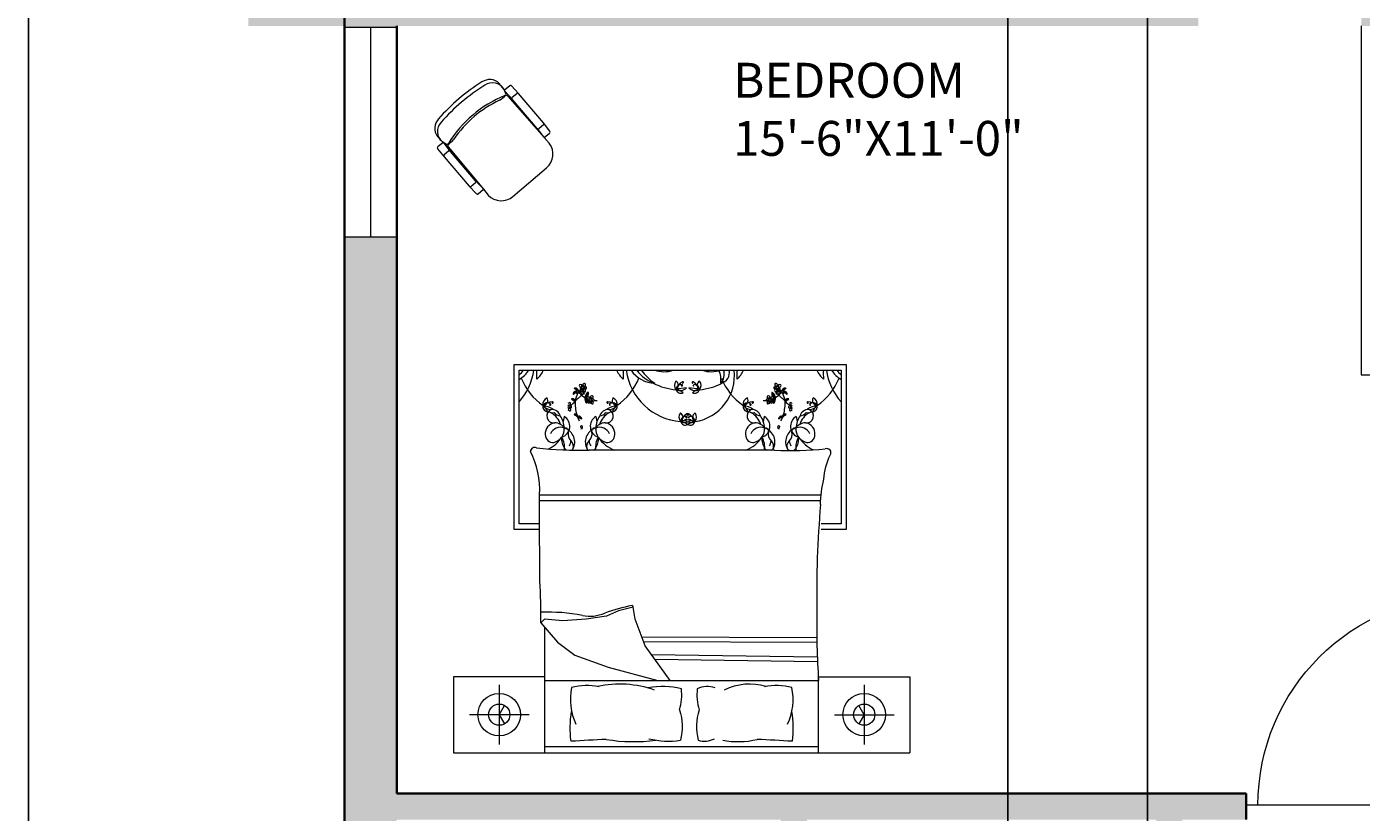
# Model space of a CAD drawing. Units: inches. Extents: x -36 to 442, y -676 to 151.
# Tile 5 of 8: x -36 to 193, y -134 to 1. Entities that reach past the tile are written whole.
import ezdxf

# ---------------------------------------------------------------- set-up
doc = ezdxf.new("R2010")
doc.units = ezdxf.units.IN
doc.header["$MEASUREMENT"] = 0
for name, color, linetype, lineweight in [('A-ANNO-DIMS', 2, 'Continuous', 18), ('A-AREA-IDEN', 7, 'Continuous', 18), ('A-DOOR', 4, 'Continuous', 18), ('A-FLOR-CASE', 32, 'Continuous', 18), ('A-FURN', 9, 'Continuous', 13), ('A-GLAZ', 4, 'Continuous', 13), ('A-WALL', 7, 'Continuous', 35), ('A-WALL-PATT', 8, 'Continuous', 13)]:
    doc.layers.add(name, color=color, linetype=linetype, lineweight=lineweight)
doc.styles.get("Standard").update_dxf_attribs({"font": 'arial.ttf'})
doc.dimstyles.get("Standard").update_dxf_attribs({"dimtxt": 0.18, "dimasz": 0.18, "dimexe": 0.18, "dimexo": 0.0625, "dimgap": 0.09, "dimtad": 0, "dimtih": 1, "dimtoh": 1, "dimdec": 0, "dimzin": 0, "dimdsep": 46, "dimlunit": 3, "dimtxsty": 'Standard', "dimcen": 0.09, "dimadec": 0, "dimazin": 0, "dimtfac": 1, "dimtdec": 0, "dimtofl": 0, "dimtmove": 0, "dimatfit": 3, "dimfxl": 1, "dimtolj": 1, "dimtzin": 0, "dimarcsym": 0})

# ---------------------------------------------------------------- blocks, each defined once
blk = doc.blocks.new('DOOR-SWING-36IN')
for p, q in [((2, 0), (2, 36)), ((3, 0), (3, 36)), ((0, 0), (2, 0)), ((2, 0), (3, 0)), ((3, 0), (38, 0)), ((38, 0), (40, 0))]:
    blk.add_line(p, q)
blk.add_arc((2, 0), 36, 0, 90)
blk = doc.blocks.new('GLAZING-UNIT-36IN')
for p, q in [((0, 36), (0, 0)), ((4.5, 36), (4.5, 0)), ((9, 0), (9, 36))]:
    blk.add_line(p, q)
blk = doc.blocks.new('*D50')
at = {"layer": 'A-ANNO-DIMS', "color": 0, "lineweight": -2, "transparency": 16777216}
for p, q in [((97.44, 113.5), (-35.74, 113.5)), ((-35.56, 113.32), (-35.56, -262.07)), ((-35.56, -637.82), (-35.56, -262.43)), ((18.67, -638), (-35.74, -638))]:
    blk.add_line(p, q, dxfattribs=at)
at = {"layer": 'A-ANNO-DIMS', "color": 0, "transparency": 16777216}
for points in [[(-35.59, 113.32), (-35.53, 113.32), (-35.56, 113.5)], [(-35.59, -637.82), (-35.53, -637.82), (-35.56, -638)]]:
    blk.add_solid(points, dxfattribs=at)
at = {"layer": 'Defpoints', "color": 0, "transparency": 16777216}
for p in [(-35.56, 113.5), (97.5, 113.5), (18.74, -638)]:
    blk.add_point(p, dxfattribs=at)
at = {"layer": 'A-ANNO-DIMS', "color": 0, "transparency": 16777216, "insert": (-35.56, -262.25), "char_height": 0.18, "attachment_point": 5}
blk.add_mtext('\\A1;751.5', dxfattribs=at)
blk = doc.blocks.new('*D63')
at = {"layer": 'A-ANNO-DIMS', "color": 0, "lineweight": -2, "transparency": 16777216}
for p, q in [((132.74, -447.43), (132.74, 151.48)), ((156.74, -471.43), (156.74, 151.48)), ((132.92, 151.3), (144.51, 151.3)), ((156.56, 151.3), (144.96, 151.3))]:
    blk.add_line(p, q, dxfattribs=at)
at = {"layer": 'A-ANNO-DIMS', "color": 0, "transparency": 16777216}
for points in [[(132.92, 151.33), (132.92, 151.27), (132.74, 151.3)], [(156.56, 151.33), (156.56, 151.27), (156.74, 151.3)]]:
    blk.add_solid(points, dxfattribs=at)
at = {"layer": 'Defpoints', "color": 0, "transparency": 16777216}
for p in [(156.74, 151.3), (132.74, -447.5), (156.74, -471.5)]:
    blk.add_point(p, dxfattribs=at)
at = {"layer": 'A-ANNO-DIMS', "color": 0, "transparency": 16777216, "insert": (144.74, 151.3), "char_height": 0.18, "attachment_point": 5}
blk.add_mtext('\\A1;24', dxfattribs=at)

msp = doc.modelspace()

# ---------------------------------------------------------------- hatches: boundary and pattern name
at = {"layer": 'A-WALL-PATT'}
h = msp.add_hatch(color=256, dxfattribs=at)
h.dxf.hatch_style = 1
h.paths.add_polyline_path([(288, 113.503), (193.5, 113.503), (97.5, 113.503), (97.5, 104.864), (106.5, 104.864), (106.5, 104.503), (193.5, 104.503), (193.5, 5.503), (193.5, 1.003), (213.735, 1.003), (213.735, -135.497), (218.235, -135.497), (218.235, 1.003), (251, 1.003), (251, 3.253), (251, 5.503), (198, 5.503), (198, 104.503), (279, 104.503), (279, 104.209), (288, 104.209)])
h.paths.add_polyline_path([(378.735, 81.646), (362.235, 81.646), (288, 81.646), (288, 80.209), (279, 80.209), (279, 5.503), (279, 1.003), (353.235, 1.003), (353.235, 0.242), (362.235, 0.242), (362.235, 5.503), (288, 5.503), (288, 77.146), (362.235, 77.146), (374.235, 77.146), (374.235, 5.503), (362.235, 5.503), (362.235, 1.003), (374.235, 1.003), (378.735, 1.003), (378.735, 5.503), (378.735, 77.146)])
h.paths.add_polyline_path([(362.235, -35.758), (353.235, -35.758), (353.235, -196.997), (218.235, -196.997), (213.735, -196.997), (213.735, -205.997), (218.235, -205.997), (378.735, -205.997), (378.735, -205.779), (387.735, -205.779), (387.735, -202.472), (387.735, -196.997), (378.735, -196.997), (362.235, -196.997)])
h.paths.add_polyline_path([(218.235, -175.497), (215.985, -175.497), (213.735, -175.497), (213.735, -196.997), (218.235, -196.997)], flags=17)
h.paths.add_polyline_path([(158.235, -201.497), (98.235, -201.497), (98.235, -205.997), (158.235, -205.997)])
h.paths.add_polyline_path([(173.735, -130.997), (27.735, -130.997), (27.735, -35.267), (18.735, -35.267), (18.735, -138.68), (27.735, -138.68), (27.735, -135.497), (93.735, -135.497), (93.735, -201.497), (98.235, -201.497), (98.235, -135.497), (158.235, -135.497), (158.235, -173.497), (160.739, -173.497), (162.735, -173.497), (162.735, -135.497), (173.735, -135.497), (173.735, -133.017)])
h.paths.add_polyline_path([(98.235, -201.497), (93.735, -201.497), (93.735, -205.997), (98.235, -205.997)])
h.paths.add_polyline_path([(162.735, -201.497), (158.235, -201.497), (158.235, -205.997), (162.735, -205.997)])
h.paths.add_polyline_path([(63.735, -205.997), (63.735, -201.497), (27.735, -201.497), (27.735, -162.68), (18.735, -162.68), (18.735, -210.497), (63.735, -210.497)])
h.paths.add_polyline_path([(65.735, -203.604), (65.735, -201.497), (63.735, -201.497), (63.735, -205.997), (65.735, -205.997)])
h.paths.add_polyline_path([(165.5, 5.503), (106.5, 5.503), (106.5, 80.864), (97.5, 80.864), (97.5, 81.646), (6.735, 81.646), (2.235, 81.646), (2.235, 77.146), (2.235, 5.503), (2.235, 1.003), (6.735, 1.003), (18.735, 1.003), (18.735, 5.503), (6.735, 5.503), (6.735, 77.146), (97.5, 77.146), (97.5, 5.503), (18.735, 5.503), (18.735, 0.733), (27.735, 0.733), (27.735, 1.003), (165.5, 1.003), (165.5, 3.253)])
h.paths.add_polyline_path([(18.735, -201.497), (6.735, -201.497), (2.235, -201.497), (2.235, -210.497), (2.235, -354.497), (2.235, -363.497), (6.735, -363.497), (18.735, -363.497), (18.735, -358.997), (18.735, -354.497), (6.735, -354.497), (6.735, -210.497), (18.735, -210.497)])
h.paths.add_polyline_path([(63.735, -210.497), (54.735, -210.497), (54.735, -240.747), (63.735, -240.747)])
h.paths.add_polyline_path([(63.735, -336.747), (54.735, -336.747), (54.735, -354.497), (18.735, -354.497), (18.735, -358.997), (18.735, -363.497), (104.735, -363.497), (104.735, -361.247), (104.735, -358.997), (63.735, -358.997)])
h.paths.add_polyline_path([(27.735, -448.151), (18.735, -448.151), (18.735, -637.997), (72.735, -637.997), (72.735, -571.997), (183.235, -571.997), (183.235, -562.997), (57.197, -562.997), (51.735, -562.997), (51.735, -567.497), (57.197, -567.497), (63.735, -567.497), (63.735, -571.997), (63.735, -628.997), (27.735, -628.997), (27.735, -475.997), (27.735, -471.497)])
h.paths.add_polyline_path([(27.735, -363.497), (18.735, -363.497), (18.735, -412.151), (27.735, -412.151)])
h.paths.add_polyline_path([(161.235, -358.997), (132.735, -358.997), (132.735, -363.497), (156.735, -363.497), (156.735, -471.497), (51.735, -471.497), (51.735, -475.997), (63.735, -475.997), (63.735, -534.997), (65.985, -534.997), (68.235, -534.997), (68.235, -475.997), (161.235, -475.997)])
h.paths.add_polyline_path([(161.235, -511.997), (173.235, -511.997), (173.235, -502.997), (161.235, -502.997), (161.235, -475.997), (152.235, -475.997), (152.235, -534.997), (156.735, -534.997), (161.235, -534.997)], flags=17)
h.paths.add_polyline_path([(362.235, -502.997), (353.235, -502.997), (213.235, -502.997), (213.235, -507.497), (213.235, -511.997), (362.235, -511.997)])
h.paths.add_polyline_path([(242.235, -548.019), (233.235, -548.019), (233.235, -562.997), (223.235, -562.997), (223.235, -567.497), (223.235, -571.997), (242.235, -571.997)])
h.paths.add_polyline_path([(404.235, -502.997), (399.735, -502.997), (362.235, -502.997), (362.235, -511.997), (399.735, -511.997), (404.235, -511.997)])
h.paths.add_polyline_path([(362.235, -482.123), (353.235, -482.123), (353.235, -502.997), (362.235, -502.997)])
h.paths.add_polyline_path([(404.235, -295.997), (404.235, -286.997), (387.735, -286.997), (387.735, -295.997), (399.735, -295.997), (399.735, -502.997), (404.235, -502.997)])
h.paths.add_polyline_path([(362.235, -355.863), (353.235, -355.863), (353.235, -386.123), (362.235, -386.123)])
h.paths.add_polyline_path([(387.735, -286.997), (378.735, -286.997), (213.735, -286.997), (213.735, -295.997), (353.235, -295.997), (353.235, -295.863), (362.235, -295.863), (362.235, -295.997), (378.735, -295.997), (387.735, -295.997)])
h.paths.add_polyline_path([(387.735, -241.779), (378.735, -241.779), (378.735, -286.997), (387.735, -286.997)])
h.paths.add_polyline_path([(387.735, -175.497), (362.235, -175.497), (362.235, -184.497), (387.735, -184.497)], flags=17)
h.paths.add_polyline_path([(387.735, -184.497), (383.235, -184.497), (383.235, -192.497), (378.735, -192.497), (366.735, -192.497), (366.735, -184.497), (362.235, -184.497), (362.235, -196.997), (378.735, -196.997), (387.735, -196.997)], flags=17)
h.paths.add_polyline_path([(240.604, 40.967), (282.575, 40.967), (282.575, 63.356), (240.604, 63.356)], flags=25)

# ---------------------------------------------------------------- linework, layer by layer
at = {"layer": 'A-FLOR-CASE'}
for p, q in [((193.5, 1.003), (193.5, -58.997)), ((193.5, -58.997), (213.735, -58.997))]:
    msp.add_line(p, q, dxfattribs=at)
at = {"layer": 'A-FURN', "ltscale": 0.03}
for p, q in [((45.926, -9.597), (45.342, -8.918)), ((46.56, -10.788), (46.166, -9.936)), ((47.561, -11.582), (46.359, -10.265)), ((46.834, -11.066), (53.081, -18.212)), ((47.587, -11.252), (48.345, -10.608)), ((51.846, -16.621), (47.561, -11.582)), ((52.934, -16.003), (52.176, -16.647)), ((35.278, -18.653), (34.702, -17.967)), ((51.846, -16.621), (52.686, -17.761)), ((36.353, -19.469), (35.575, -18.944)), ((36.975, -20.585), (35.868, -19.188)), ((36.645, -20.558), (35.888, -21.203)), ((36.583, -19.785), (42.633, -27.098)), ((41.261, -25.624), (36.975, -20.585)), ((40.476, -26.598), (41.234, -25.954)), ((41.261, -25.624), (42.251, -26.636))]:
    msp.add_line(p, q, dxfattribs=at)
at = {"layer": 'A-FURN'}
for p, q in [((47.849, -57.313), (47.849, -85.559)), ((105.014, -57.313), (47.849, -57.313)), ((105.014, -85.559), (105.014, -57.313)), ((48.757, -58.221), (104.105, -58.221)), ((48.757, -84.65), (48.757, -58.221)), ((104.105, -58.221), (104.105, -84.65)), ((56.484, -66.171), (56.311, -67.057)), ((61.964, -66.171), (62.138, -67.057)), ((90.898, -66.171), (90.725, -67.057)), ((96.378, -66.171), (96.551, -67.057)), ((92.623, -71.988), (60.787, -71.988)), ((100.659, -79.69), (52.278, -79.69)), ((100.584, -80.668), (52.278, -80.668)), ((52.282, -84.65), (48.757, -84.65)), ((104.105, -84.65), (100.649, -84.65)), ((47.849, -85.559), (52.284, -85.559)), ((100.665, -85.559), (105.014, -85.559)), ((63.755, -100.545), (60.261, -101.021)), ((65.82, -99.593), (63.755, -100.545)), ((68.361, -98.958), (65.82, -99.593)), ((68.679, -101.021), (68.361, -98.958)), ((53.115, -101.021), (52.479, -101.656)), ((52.479, -101.656), (55.338, -104.989)), ((56.291, -101.339), (53.115, -101.021)), ((53.181, -123.996), (53.181, -102.475)), ((60.261, -101.021), (56.291, -101.339)), ((70.426, -105.624), (68.679, -101.021)), ((55.338, -104.989), (58.356, -107.211)), ((99.951, -104.269), (69.865, -104.146)), ((99.947, -105.074), (70.172, -104.956)), ((58.356, -107.211), (64.073, -109.275)), ((74.722, -111.605), (70.426, -105.624)), ((99.987, -107.543), (71.515, -107.141)), ((64.073, -109.275), (72.623, -111.605)), ((100.018, -108.348), (72.101, -107.956)), ((45.34, -112.339), (45.34, -122.585)), ((53.181, -111.605), (100.228, -111.605)), ((108.069, -112.339), (108.069, -122.585)), ((50.463, -117.462), (40.217, -117.462)), ((102.946, -117.462), (113.192, -117.462)), ((100.228, -122.99), (53.181, -122.99)), ((37.499, -123.996), (115.91, -123.996))]:
    msp.add_line(p, q, dxfattribs=at)
at = {"layer": 'A-FURN', "ltscale": 0.03}
msp.add_lwpolyline([(34.702, -17.967), (34.99, -18.31, 0.029912), (35.457, -18.852, 0.0631929), (35.697, -19.026), (34.781, -19.805, 0.4142136), (34.754, -20.135), (35.861, -21.533), (40.146, -26.571), (40.146, -26.571), (40.146, -26.571), (41.393, -27.845, 0.4142136), (41.723, -27.872), (42.633, -27.098), (43.458, -28.095, 0.4039906), (47.693, -28.333), (53.488, -23.405, 0.4039906), (53.932, -19.186), (53.081, -18.212), (53.991, -17.438, 0.4142136), (54.018, -17.108), (52.96, -15.673), (48.675, -10.634), (47.473, -9.318, 0.4142136), (47.143, -9.291), (46.227, -10.07, 0.0631952), (46.094, -9.806, 0.029912), (45.634, -9.257), (45.342, -8.918, 0.1969574), (43.912, -8.235, 0.1563962), (42.376, -8.633, 0.0348091), (38.409, -11.547, 0.0348091), (34.897, -14.994, 0.1563962), (34.258, -16.446, 0.1969574)], format="xyb", close=True, dxfattribs=at)
at = {"layer": 'A-FURN'}
for points in [[(52.315, -94.476, -0.0012423), (52.278, -79.599, 0.1272016), (50.706, -72.184)], [(100.563, -81.286, -0.0561118), (101.132, -76.972, -0.0953413), (102.234, -72.816)], [(57.685, -122.042, -0.0748968), (57.78, -116.92, 0.4728166)], [(76.337, -116.634, -0.1409896), (76.494, -121.859, -0.2352448)], [(79.686, -116.634, 0.1409896), (79.529, -121.859, 0.2352448)], [(95.724, -122.042, 0.0748968), (95.629, -116.92, -0.4728166)]]:
    msp.add_lwpolyline(points, format="xyb", dxfattribs=at)
for points in [[(53.181, -110.928), (37.499, -110.928), (37.499, -123.996)], [(100.228, -123.996), (100.228, -110.928), (115.91, -110.928), (115.91, -123.996)], [(45.34, -117.462), (46.255, -115.878)], [(108.069, -117.462), (107.154, -115.878)], [(45.34, -117.462), (46.255, -119.046)], [(108.069, -117.462), (107.154, -119.046)]]:
    msp.add_lwpolyline(points, dxfattribs=at)
for centre, radius in [((59.708, -61.225), 0.2), ((93.154, -61.225), 0.2), ((61.014, -63.33), 0.2), ((91.848, -63.33), 0.2), ((45.34, -117.462), 3.659), ((108.069, -117.462), 3.659), ((45.34, -117.462), 1.83), ((108.069, -117.462), 1.83)]:
    msp.add_circle(centre, radius, dxfattribs=at)
at = {"layer": 'A-FURN', "ltscale": 0.03}
for centre, radius, start, end in [((44.163, -11.096), 2.314, 30.08252, 124.53168), ((61.256, -38.41), 34.534, 122.20561, 138.55381), ((53.845, -29.695), 20.169, 111.96244, 148.79994), ((43.335, -8.119), 4.205, 299.29135, 318.21611), ((46.281, -10.698), 0.293, 274.06172, 341.95455), ((46.527, -11.322), 0.399, 39.82995, 99.60618), ((47.739, -11.43), 0.234, 130.38119, 220.38119), ((48.497, -10.786), 0.234, 40.38119, 130.38119), ((53.845, -29.695), 19.803, 115.26646, 145.49592), ((37.041, -17.154), 2.314, 136.2307, 230.67985), ((52.782, -15.825), 0.234, 310.38119, 40.38119), ((52.024, -16.469), 0.234, 220.38119, 310.38119), ((36.308, -19.18), 0.293, 278.80783, 346.70066), ((36.884, -19.523), 0.399, 161.15619, 220.93242), ((34.235, -15.858), 4.205, 302.54626, 321.47102), ((36.797, -20.737), 0.234, 40.38119, 130.38119), ((36.039, -21.381), 0.234, 130.38119, 220.38119), ((40.325, -26.42), 0.234, 220.38119, 310.38119), ((41.082, -25.775), 0.234, 310.38119, 40.38119)]:
    msp.add_arc(centre, radius, start, end, dxfattribs=at)
at = {"layer": 'A-FURN'}
for centre, radius, start, end in [((44.476, -54.54), 6.218, 313.51858, 323.69643), ((46.271, -55.47), 4.989, 299.88843, 326.53828), ((41.134, -56.842), 10.239, 318.1144, 352.25504), ((58.652, -55.829), 10.239, 201.40921, 235.61345), ((49.065, -56.625), 4.163, 311.04544, 337.44526), ((37.661, -58.862), 14.167, 356.34809, 2.59189), ((69.383, -56.625), 4.163, 202.55474, 228.95456), ((59.796, -55.829), 10.239, 304.38655, 338.59079), ((80.787, -58.862), 14.167, 177.40811, 183.65191), ((77.314, -56.842), 10.239, 187.74496, 265.53767), ((72.178, -55.47), 4.989, 213.46172, 268.72803), ((73.973, -54.54), 6.218, 216.30357, 252.14962), ((77.24, -52.792), 9.249, 215.94696, 235.98766), ((73.667, -52.838), 5.63, 252.9798, 286.45689), ((75.897, -49.936), 8.326, 264.36426, 265.62128), ((80.283, -44.232), 14.878, 250.09716, 250.27829), ((77.831, -59.206), 7.925, 278.18034, 7.13645), ((81.809, -52.838), 5.63, 253.54311, 287.0202), ((79.579, -49.936), 8.326, 274.37872, 275.63574), ((75.194, -44.232), 14.878, 289.72171, 289.90284), ((78.855, -59.93), 4.584, 353.38046, 21.88297), ((83.061, -58.654), 1.838, 280.92615, 13.61018), ((81.68, -58.906), 2.324, 318.09513, 17.13912), ((93.066, -55.829), 10.239, 201.40921, 235.61345), ((72.075, -58.862), 14.167, 356.34809, 2.59189), ((83.479, -56.625), 4.163, 311.04544, 337.44526), ((103.797, -56.625), 4.163, 202.55474, 228.95456), ((94.21, -55.829), 10.239, 304.38655, 338.59079), ((115.201, -58.862), 14.167, 177.40811, 183.65191), ((111.728, -56.842), 10.239, 187.74496, 221.8856), ((106.591, -55.47), 4.989, 213.46172, 240.11157), ((108.387, -54.54), 6.218, 216.30357, 226.48142), ((58.57, -62.34), 0.52, 82.60083, 147.18452), ((58.42, -61.516), 0.223, 55.60767, 145.6462), ((58.268, -61.993), 0.604, 21.70871, 93.02993), ((55.086, -66.301), 5.834, 53.62539, 57.3216), ((58.453, -61.843), 0.52, 342.8042, 79.69432), ((58.409, -61.789), 0.231, 338.24522, 53.62539), ((58.785, -61.939), 0.174, 158.24522, 340.63946), ((62.06, -60.483), 3.478, 201.70871, 206.21806), ((61.649, -63.832), 3.256, 137.50829, 145.99666), ((59.384, -62.34), 0.553, 61.18377, 141.67918), ((59.289, -60.85), 0.198, 134.37319, 211.9501), ((59.655, -60.622), 0.63, 211.9501, 255.24419), ((59.302, -61.072), 0.394, 8.56141, 112.59143), ((59.488, -61.503), 0.272, 88.57189, 233.89544), ((59.457, -61.577), 0.196, 228.29465, 6.24744), ((59.412, -61.056), 0.132, 352.86802, 97.09399), ((59.273, -61.344), 0.275, 298.84925, 359.93549), ((59.339, -61.578), 0.314, 4.21229, 48.15875), ((59.98, -60.855), 0.33, 100.95974, 208.78041), ((59.343, -62.441), 0.661, 15.64837, 62.29574), ((59.984, -61.534), 0.333, 183.63497, 258.43627), ((59.941, -61.414), 0.191, 178.13253, 268.89195), ((60.336, -61.294), 0.606, 132.38963, 156.57243), ((60.069, -61.372), 0.327, 42.32085, 130.21108), ((60.144, -61.03), 0.413, 226.34618, 279.6513), ((59.717, -61.795), 0.48, 7.49685, 71.27373), ((59.701, -60.68), 0.464, 291.63824, 4.94696), ((60.065, -60.601), 0.654, 254.28291, 276.91484), ((60.011, -60.653), 0.153, 4.94696, 127.52629), ((60.044, -61.772), 0.154, 215.0752, 14.76444), ((60.184, -61.268), 0.172, 279.6513, 42.32085), ((76.53, -51.357), 10.239, 242.5854, 265.53767), ((76.575, -60.803), 1.135, 140.88554, 222.21268), ((75.285, -60.837), 0.855, 301.63732, 61.4609), ((76.571, -61.533), 0.838, 76.14802, 182.24151), ((78.183, -62.405), 2.59, 121.98902, 161.08405), ((77.877, -68.401), 7.163, 92.74183, 107.40696), ((76.4, -60.09), 1.619, 245.68992, 314.45887), ((75.689, -63.314), 1.749, 44.62734, 88.54154), ((76.549, -61.329), 0.849, 196.19625, 296.97263), ((76.745, -60.827), 0.111, 140.07546, 76.14802), ((76.879, -60.317), 0.127, 288.44082, 121.98902), ((76.9, -60.379), 0.0618, 171.98332, 288.44082), ((77.599, -68.401), 7.163, 72.59304, 87.25817), ((79.076, -60.09), 1.619, 225.54113, 294.31008), ((78.597, -60.317), 0.127, 58.01098, 251.55918), ((79.787, -63.314), 1.749, 91.45846, 135.37266), ((78.927, -61.329), 0.849, 243.02737, 343.80375), ((78.576, -60.379), 0.0618, 251.55918, 8.01668), ((78.721, -60.87), 0.0667, 103.97912, 39.80908), ((77.293, -62.405), 2.59, 18.91595, 58.01098), ((78.905, -61.533), 0.838, 357.75849, 103.85198), ((80.191, -60.837), 0.855, 118.5391, 238.36268), ((78.901, -60.803), 1.135, 317.78732, 39.11446), ((78.946, -51.357), 10.239, 274.46233, 297.4146), ((92.679, -61.268), 0.172, 137.67915, 260.3487), ((92.793, -61.372), 0.327, 49.78892, 137.67915), ((92.719, -61.03), 0.413, 260.3487, 313.65382), ((92.819, -61.772), 0.154, 165.23556, 324.9248), ((93.145, -61.795), 0.48, 108.72627, 172.50315), ((93.161, -60.68), 0.464, 175.05304, 248.36176), ((92.852, -60.653), 0.153, 52.47371, 175.05304), ((92.797, -60.601), 0.654, 263.08516, 285.71709), ((93.519, -62.441), 0.661, 117.70426, 164.35163), ((92.921, -61.414), 0.191, 271.10805, 1.86747), ((92.526, -61.294), 0.606, 23.42757, 47.61037), ((92.882, -60.855), 0.33, 331.21959, 79.04026), ((92.878, -61.534), 0.333, 281.56373, 356.36503), ((93.561, -61.072), 0.394, 67.40857, 171.43859), ((93.405, -61.577), 0.196, 173.75256, 311.70535), ((93.524, -61.578), 0.314, 131.84125, 175.78771), ((93.479, -62.34), 0.553, 38.32082, 118.81623), ((93.589, -61.344), 0.275, 180.06451, 241.15075), ((93.45, -61.056), 0.132, 82.90601, 187.13198), ((93.208, -60.622), 0.63, 284.75581, 328.0499), ((93.375, -61.503), 0.272, 306.10456, 91.42811), ((91.213, -63.832), 3.256, 34.00334, 42.49171), ((93.574, -60.85), 0.198, 328.0499, 45.62681), ((94.409, -61.843), 0.52, 100.30568, 197.1958), ((94.077, -61.939), 0.174, 199.36054, 21.75478), ((90.802, -60.483), 3.478, 333.78194, 338.29129), ((94.594, -61.993), 0.604, 86.97007, 158.29129), ((94.453, -61.789), 0.231, 126.37461, 201.75478), ((94.292, -62.34), 0.52, 32.81548, 97.39917), ((94.442, -61.516), 0.223, 34.3538, 124.39233), ((97.776, -66.301), 5.834, 122.6784, 126.37461), ((53.979, -64.038), 1.135, 110.96132, 192.28847), ((52.844, -63.424), 0.855, 271.71311, 31.53669), ((54.574, -66.229), 2.59, 92.0648, 131.15983), ((53.611, -64.668), 0.838, 46.22381, 152.3173), ((54.114, -64.144), 0.111, 110.28165, 46.22381), ((54.472, -63.832), 0.0618, 142.05911, 258.5166), ((54.485, -63.768), 0.127, 258.5166, 92.0648), ((57.415, -64.147), 0.33, 100.95974, 142.23791), ((57.771, -64.586), 0.606, 132.38963, 156.57243), ((57.136, -63.971), 0.464, 291.63824, 4.94696), ((57.446, -63.945), 0.153, 4.94696, 127.52629), ((52.973, -58.47), 7.445, 307.9541, 316.84587), ((57.809, -65.355), 2.211, 82.86976, 91.67361), ((58.116, -62.968), 0.412, 205.53786, 258.67439), ((57.524, -64.365), 1.239, 59.34401, 79.74122), ((58.255, -62.245), 0.223, 123.09787, 213.13641), ((57.256, -64.361), 1.26, 43.69288, 51.78988), ((58.638, -62.569), 0.604, 92.31716, 160.52013), ((61.399, -67.157), 5.834, 121.11559, 124.8118), ((58.029, -63.534), 0.376, 355.71315, 81.65678), ((57.821, -63.864), 0.657, 27.36586, 59.34401), ((58.315, -63.43), 0.16, 202.55835, 304.23425), ((58.504, -62.36), 0.231, 45.73542, 121.11559), ((64.884, -63.995), 6.494, 176.17232, 196.41582), ((61.649, -63.832), 3.256, 150.79592, 175.24398), ((66.336, -70.764), 10.714, 127.82556, 137.75876), ((58.786, -62.07), 0.174, 225.73542, 48.12966), ((59.292, -62.859), 0.91, 40.93647, 112.76952), ((58.992, -62.553), 0.536, 49.38119, 95.54564), ((61.984, -59.507), 3.905, 220.18202, 239.45598), ((59.76, -61.658), 0.644, 229.38119, 289.99593), ((59.972, -63.423), 0.553, 3.87739, 87.15012), ((59.722, -62.01), 0.91, 287.88895, 359.722), ((59.694, -62.438), 0.536, 305.11283, 351.27729), ((59.581, -63.208), 0.536, 352.07481, 38.23927), ((59.486, -63.626), 0.91, 343.63009, 55.46314), ((60.749, -63.371), 0.644, 172.07481, 232.68955), ((60.13, -62.344), 0.553, 271.4625, 339.4747), ((60.86, -62.617), 0.644, 110.66254, 171.27729), ((59.865, -63.443), 0.661, 318.34199, 4.98936), ((60.595, -62.955), 0.198, 134.37319, 211.9501), ((61.984, -59.507), 3.905, 246.15226, 246.94993), ((60.961, -62.726), 0.63, 211.9501, 255.24419), ((60.608, -63.177), 0.394, 8.56141, 112.59143), ((60.794, -63.607), 0.272, 88.57189, 233.89544), ((60.033, -62.294), 0.661, 338.36273, 25.0101), ((60.764, -63.681), 0.196, 228.29465, 6.24744), ((60.719, -63.161), 0.132, 352.86802, 97.09399), ((60.58, -63.449), 0.275, 298.84925, 359.93549), ((60.645, -63.683), 0.314, 4.21229, 48.15875), ((61.286, -62.96), 0.33, 100.95974, 208.78041), ((61.29, -63.639), 0.333, 183.63497, 258.43627), ((61.247, -63.519), 0.191, 178.13253, 268.89195), ((61.642, -63.399), 0.606, 132.38963, 156.57243), ((61.376, -63.477), 0.327, 42.32085, 130.21108), ((61.45, -63.135), 0.413, 226.34618, 279.6513), ((61.023, -63.9), 0.48, 7.49685, 71.27373), ((61.007, -62.785), 0.464, 291.63824, 4.94696), ((61.371, -62.706), 0.654, 254.28291, 276.91484), ((61.317, -62.758), 0.153, 4.94696, 127.52629), ((61.35, -63.877), 0.154, 215.0752, 14.76444), ((61.49, -63.372), 0.172, 279.6513, 42.32085), ((61.984, -59.507), 3.905, 265.24147, 272.89291), ((63.964, -63.768), 0.127, 87.9352, 281.4834), ((63.875, -66.229), 2.59, 48.84017, 87.9352), ((63.977, -63.832), 0.0618, 281.4834, 37.94089), ((64.838, -64.668), 0.838, 27.6827, 133.77619), ((64.347, -64.186), 0.0667, 133.77292, 69.73329), ((65.605, -63.424), 0.855, 148.46331, 268.28689), ((64.47, -64.038), 1.135, 347.71153, 69.03868), ((88.393, -64.038), 1.135, 110.96132, 192.28847), ((87.258, -63.424), 0.855, 271.71311, 31.53669), ((88.987, -66.229), 2.59, 92.0648, 131.15983), ((88.025, -64.668), 0.838, 46.22381, 152.3173), ((88.528, -64.144), 0.111, 110.28165, 46.22381), ((88.886, -63.832), 0.0618, 142.05911, 258.5166), ((88.899, -63.768), 0.127, 258.5166, 92.0648), ((90.878, -59.507), 3.905, 267.10709, 274.75853), ((91.372, -63.372), 0.172, 137.67915, 260.3487), ((91.487, -63.477), 0.327, 49.78892, 137.67915), ((91.413, -63.135), 0.413, 260.3487, 313.65382), ((91.512, -63.877), 0.154, 165.23556, 324.9248), ((91.839, -63.9), 0.48, 108.72627, 172.50315), ((91.855, -62.785), 0.464, 175.05304, 248.36176), ((91.545, -62.758), 0.153, 52.47371, 175.05304), ((91.491, -62.706), 0.654, 263.08516, 285.71709), ((91.615, -63.519), 0.191, 271.10805, 1.86747), ((91.22, -63.399), 0.606, 23.42757, 47.61037), ((91.576, -62.96), 0.33, 331.21959, 79.04026), ((91.572, -63.639), 0.333, 281.56373, 356.36503), ((92.255, -63.177), 0.394, 67.40857, 171.43859), ((92.099, -63.681), 0.196, 173.75256, 311.70535), ((92.218, -63.683), 0.314, 131.84125, 175.78771), ((92.283, -63.449), 0.275, 180.06451, 241.15075), ((92.144, -63.161), 0.132, 82.90601, 187.13198), ((91.901, -62.726), 0.63, 284.75581, 328.0499), ((92.069, -63.607), 0.272, 306.10456, 91.42811), ((92.829, -62.294), 0.661, 154.9899, 201.63727), ((92.733, -62.344), 0.553, 200.5253, 268.5375), ((93.14, -62.01), 0.91, 180.278, 252.11105), ((92.003, -62.617), 0.644, 8.72271, 69.33746), ((92.998, -63.443), 0.661, 175.01064, 221.65801), ((92.891, -63.423), 0.553, 92.84988, 176.12261), ((92.268, -62.955), 0.198, 328.0499, 45.62681), ((90.878, -59.507), 3.905, 293.05007, 293.84774), ((93.377, -63.626), 0.91, 124.53686, 196.36991), ((92.113, -63.371), 0.644, 307.31045, 7.92519), ((93.169, -62.438), 0.536, 188.72271, 234.88717), ((93.281, -63.208), 0.536, 141.76073, 187.92519), ((90.878, -59.507), 3.905, 300.54402, 319.81798), ((93.57, -62.859), 0.91, 67.23048, 139.06353), ((93.103, -61.658), 0.644, 250.00407, 310.61881), ((86.526, -70.764), 10.714, 42.24124, 52.17444), ((93.871, -62.553), 0.536, 84.45436, 130.61881), ((94.076, -62.07), 0.174, 131.87034, 314.26458), ((91.213, -63.832), 3.256, 4.75602, 29.20408), ((94.359, -62.36), 0.231, 58.88441, 134.26458), ((87.978, -63.995), 6.494, 343.58418, 3.82768), ((94.225, -62.569), 0.604, 19.47987, 87.68284), ((94.833, -63.534), 0.376, 98.34322, 184.28685), ((95.041, -63.864), 0.657, 120.65599, 152.63414), ((94.548, -63.43), 0.16, 235.76575, 337.44165), ((99.889, -58.47), 7.445, 223.15413, 232.0459), ((91.463, -67.157), 5.834, 55.1882, 58.88441), ((95.606, -64.361), 1.26, 128.21012, 136.30712), ((95.338, -64.365), 1.239, 100.25878, 120.65599), ((94.607, -62.245), 0.223, 326.86359, 56.90213), ((95.053, -65.355), 2.211, 88.32639, 97.13024), ((94.746, -62.968), 0.412, 281.32561, 334.46214), ((95.726, -63.971), 0.464, 175.05304, 248.36176), ((95.417, -63.945), 0.153, 52.47371, 175.05304), ((95.091, -64.586), 0.606, 23.42757, 47.61037), ((95.447, -64.147), 0.33, 37.76209, 79.04026), ((98.377, -63.768), 0.127, 87.9352, 281.4834), ((98.289, -66.229), 2.59, 48.84017, 87.9352), ((98.39, -63.832), 0.0618, 281.4834, 37.94089), ((99.251, -64.668), 0.838, 27.6827, 133.77619), ((98.761, -64.186), 0.0667, 133.77292, 69.73329), ((100.019, -63.424), 0.855, 148.46331, 268.28689), ((98.884, -64.038), 1.135, 347.71153, 69.03868), ((53.694, -64.481), 0.849, 166.27204, 267.04841), ((51.317, -71.272), 7.163, 62.81761, 77.48274), ((54.183, -63.333), 1.619, 215.76571, 284.53465), ((51.959, -65.772), 1.749, 14.70312, 58.61733), ((54.691, -66.107), 1.177, 109.13116, 279.73602), ((54.449, -64.832), 0.721, 216.73195, 296.02445), ((52.358, -68.698), 3.702, 18.2955, 58.73863), ((54.408, -66.461), 1.47, 15.6955, 94.03098), ((55.991, -64.508), 1.565, 218.41745, 263.8338), ((52.323, -68.399), 4.208, 3.4924, 33.71172), ((55.512, -67.861), 1.949, 286.8663, 60.09146), ((57.143, -64.516), 0.2, 273.27684, 86.72316), ((57.419, -64.826), 0.333, 217.3642, 258.43627), ((57.376, -64.705), 0.191, 178.13253, 268.89195), ((57.504, -64.663), 0.327, 42.32085, 130.21108), ((57.578, -64.322), 0.413, 226.34618, 279.6513), ((57.152, -65.087), 0.48, 7.49685, 71.27373), ((57.5, -63.893), 0.654, 254.28291, 276.91484), ((57.479, -65.063), 0.154, 215.0752, 14.76444), ((57.619, -64.559), 0.172, 279.6513, 42.32085), ((58.277, -67.994), 2.211, 82.86976, 91.67361), ((58.583, -65.606), 0.412, 205.53786, 258.67439), ((57.991, -67.003), 1.239, 59.34401, 79.74122), ((57.723, -67), 1.26, 43.69288, 51.78988), ((58.496, -66.172), 0.376, 355.71315, 81.65678), ((58.288, -66.502), 0.657, 27.36586, 59.34401), ((58.782, -66.068), 0.16, 202.55835, 304.23425), ((64.884, -63.995), 6.494, 200.10592, 206.9968), ((59.031, -66.217), 0.16, 173.94573, 275.62162), ((59.074, -66.518), 0.376, 36.52319, 122.46683), ((58.881, -66.857), 0.657, 58.83597, 90.81412), ((58.709, -67.59), 1.26, 66.39009, 74.48709), ((59.531, -66.174), 0.412, 219.50559, 272.64212), ((58.58, -67.355), 1.239, 38.43876, 58.83597), ((57.572, -67.572), 2.211, 26.50636, 35.31021), ((62.936, -67.861), 1.949, 119.90854, 253.1337), ((66.126, -68.399), 4.208, 146.28828, 176.5076), ((66.091, -68.698), 3.702, 121.26137, 161.7045), ((64.04, -66.461), 1.47, 85.96902, 164.3045), ((62.457, -64.508), 1.565, 276.1662, 321.58255), ((63.758, -66.107), 1.177, 260.26398, 70.86884), ((64, -64.832), 0.721, 243.97555, 323.26805), ((64.266, -63.333), 1.619, 255.46535, 324.23429), ((67.132, -71.272), 7.163, 102.51726, 117.18239), ((64.755, -64.481), 0.849, 272.95159, 13.72796), ((66.49, -65.772), 1.749, 121.38267, 165.29688), ((77.359, -66.287), 1.135, 140.88554, 222.21268), ((76.069, -66.322), 0.855, 301.63732, 61.4609), ((77.355, -67.017), 0.838, 76.14802, 182.24151), ((78.967, -67.889), 2.59, 121.98902, 161.08405), ((77.529, -66.311), 0.111, 140.07546, 76.14802), ((77.663, -65.801), 0.127, 288.44082, 121.98902), ((77.684, -65.863), 0.0618, 171.98332, 288.44082), ((77.813, -65.801), 0.127, 58.01098, 251.55918), ((77.792, -65.863), 0.0618, 251.55918, 8.01668), ((77.937, -66.354), 0.0667, 103.97912, 39.80908), ((76.509, -67.889), 2.59, 18.91595, 58.01098), ((78.121, -67.017), 0.838, 357.75849, 103.85198), ((79.407, -66.322), 0.855, 118.5391, 238.36268), ((78.117, -66.287), 1.135, 317.78732, 39.11446), ((88.108, -64.481), 0.849, 166.27204, 267.04841), ((86.372, -65.772), 1.749, 14.70312, 58.61733), ((88.597, -63.333), 1.619, 215.76571, 284.53465), ((85.731, -71.272), 7.163, 62.81761, 77.48274), ((89.105, -66.107), 1.177, 109.13116, 279.73602), ((88.862, -64.832), 0.721, 216.73195, 296.02445), ((86.771, -68.698), 3.702, 18.2955, 58.73863), ((88.822, -66.461), 1.47, 15.6955, 94.03098), ((90.405, -64.508), 1.565, 218.41745, 263.8338), ((86.737, -68.399), 4.208, 3.4924, 33.71172), ((89.926, -67.861), 1.949, 286.8663, 60.09146), ((95.291, -67.572), 2.211, 144.68979, 153.49364), ((94.283, -67.355), 1.239, 121.16403, 141.56124), ((93.331, -66.174), 0.412, 267.35788, 320.49441), ((93.789, -66.518), 0.376, 57.53317, 143.47681), ((93.981, -66.857), 0.657, 89.18588, 121.16403), ((94.153, -67.59), 1.26, 105.51291, 113.60991), ((87.978, -63.995), 6.494, 333.0032, 339.89408), ((93.832, -66.217), 0.16, 264.37838, 6.05427), ((94.366, -66.172), 0.376, 98.34322, 184.28685), ((94.574, -66.502), 0.657, 120.65599, 152.63414), ((94.081, -66.068), 0.16, 235.76575, 337.44165), ((95.139, -67), 1.26, 128.21012, 136.30712), ((94.871, -67.003), 1.239, 100.25878, 120.65599), ((94.586, -67.994), 2.211, 88.32639, 97.13024), ((94.279, -65.606), 0.412, 281.32561, 334.46214), ((95.244, -64.559), 0.172, 137.67915, 260.3487), ((95.358, -64.663), 0.327, 49.78892, 137.67915), ((95.284, -64.322), 0.413, 260.3487, 313.65382), ((95.384, -65.063), 0.154, 165.23556, 324.9248), ((95.71, -65.087), 0.48, 108.72627, 172.50315), ((95.362, -63.893), 0.654, 263.08516, 285.71709), ((97.35, -67.861), 1.949, 119.90854, 253.1337), ((95.486, -64.705), 0.191, 271.10805, 1.86747), ((95.443, -64.826), 0.333, 281.56373, 322.6358), ((95.719, -64.516), 0.2, 93.27684, 266.72316), ((100.539, -68.399), 4.208, 146.28828, 176.5076), ((100.505, -68.698), 3.702, 121.26137, 161.7045), ((98.454, -66.461), 1.47, 85.96902, 164.3045), ((96.871, -64.508), 1.565, 276.1662, 321.58255), ((98.172, -66.107), 1.177, 260.26398, 70.86884), ((98.414, -64.832), 0.721, 243.97555, 323.26805), ((101.546, -71.272), 7.163, 102.51726, 117.18239), ((98.68, -63.333), 1.619, 255.46535, 324.23429), ((100.904, -65.772), 1.749, 121.38267, 165.29688), ((99.168, -64.481), 0.849, 272.95159, 13.72796), ((55.122, -69.127), 1.874, 97.11425, 185.05515), ((55.858, -69.837), 1.82, 68.57785, 158.41813), ((54.173, -68.337), 2.358, 283.079, 4.70666), ((54.796, -69.543), 2.278, 35.95986, 87.6409), ((59.075, -69.998), 3.024, 143.65552, 147.29887), ((56.747, -68.68), 0.487, 344.85287, 102.69594), ((55.815, -70.564), 2.499, 330.8249, 70.71782), ((58.768, -69.227), 1.608, 164.85287, 228.43469), ((59.449, -67.942), 0.151, 79.56155, 257.29493), ((59.432, -68.035), 0.246, 259.58644, 79.56155), ((62.634, -70.564), 2.499, 109.28218, 209.1751), ((59.681, -69.227), 1.608, 311.56531, 15.14713), ((61.702, -68.68), 0.487, 77.30406, 195.14713), ((63.653, -69.543), 2.278, 92.3591, 144.04014), ((59.373, -69.998), 3.024, 32.70113, 36.34448), ((64.276, -68.337), 2.358, 175.29334, 256.921), ((62.59, -69.837), 1.82, 21.58187, 111.42215), ((63.327, -69.127), 1.874, 354.94485, 82.88575), ((77.184, -65.575), 1.619, 245.68992, 314.45887), ((78.661, -73.885), 7.163, 92.74183, 107.40696), ((77.333, -66.813), 0.849, 196.19625, 296.97263), ((76.473, -68.798), 1.749, 44.62734, 88.54154), ((78.292, -65.575), 1.619, 225.54113, 294.31008), ((76.816, -73.885), 7.163, 72.59304, 87.25817), ((78.143, -66.813), 0.849, 243.02737, 343.80375), ((79.003, -68.798), 1.749, 91.45846, 135.37266), ((89.536, -69.127), 1.874, 97.11425, 185.05515), ((90.272, -69.837), 1.82, 68.57785, 158.41813), ((88.586, -68.337), 2.358, 283.079, 4.70666), ((89.21, -69.543), 2.278, 35.95986, 87.6409), ((93.489, -69.998), 3.024, 143.65552, 147.29887), ((91.16, -68.68), 0.487, 344.85287, 102.69594), ((90.228, -70.564), 2.499, 330.8249, 70.71782), ((93.182, -69.227), 1.608, 164.85287, 228.43469), ((93.43, -68.035), 0.246, 100.43845, 280.41356), ((93.413, -67.942), 0.151, 282.70507, 100.43845), ((97.048, -70.564), 2.499, 109.28218, 209.1751), ((94.094, -69.227), 1.608, 311.56531, 15.14713), ((96.116, -68.68), 0.487, 77.30406, 195.14713), ((98.066, -69.543), 2.278, 92.3591, 144.04014), ((93.787, -69.998), 3.024, 32.70113, 36.34448), ((98.69, -68.337), 2.358, 175.29334, 256.921), ((97.004, -69.837), 1.82, 21.58187, 111.42215), ((97.741, -69.127), 1.874, 354.94485, 82.88575), ((54.579, -69.316), 1.324, 178.94622, 275.51443), ((51.122, -66.466), 5.935, 296.70034, 326.33288), ((59.075, -69.998), 3.024, 175.26963, 214.21495), ((53.299, -71.408), 3.249, 350.84458, 31.17822), ((55.437, -70.112), 2.254, 330.08513, 352.56401), ((56.923, -71.308), 1.173, 336.16459, 48.43469), ((61.526, -71.308), 1.173, 131.56531, 203.83541), ((63.011, -70.112), 2.254, 187.43599, 209.91487), ((59.373, -69.998), 3.024, 325.78505, 4.73037), ((65.15, -71.408), 3.249, 148.82178, 190.28665), ((67.327, -66.466), 5.935, 213.66712, 248.50587), ((63.87, -69.316), 1.324, 264.48557, 1.05378), ((88.993, -69.316), 1.324, 178.94622, 275.51443), ((85.536, -66.466), 5.935, 291.49413, 326.33288), ((93.489, -69.998), 3.024, 175.26963, 214.21495), ((87.712, -71.408), 3.249, 349.71335, 31.17822), ((89.851, -70.112), 2.254, 330.08513, 352.56401), ((91.337, -71.308), 1.173, 336.16459, 48.43469), ((95.939, -71.308), 1.173, 131.56531, 203.83541), ((97.425, -70.112), 2.254, 187.43599, 209.91487), ((93.787, -69.998), 3.024, 325.78505, 4.73037), ((99.564, -71.408), 3.249, 148.82178, 190.75101), ((101.741, -66.466), 5.935, 213.66712, 246.35467), ((98.283, -69.316), 1.324, 264.48557, 1.05378), ((51.428, -72.234), 0.724, 62.65876, 176.02002), ((59.851, 9.633), 81.627, 264.31131, 270.65675), ((57.322, -71.121), 0.944, 217.67503, 239.9707), ((57.322, -71.121), 0.944, 296.44199, 315.54831), ((61.126, -71.121), 0.944, 224.45169, 246.77099), ((61.126, -71.121), 0.944, 293.28564, 322.32497), ((91.736, -71.121), 0.944, 217.67503, 246.71436), ((91.736, -71.121), 0.944, 293.28564, 315.54831), ((95.024, 4.274), 76.3, 268.19649, 274.75976), ((95.54, -71.121), 0.944, 224.45169, 253.36566), ((95.54, -71.121), 0.944, 287.41857, 322.32497), ((101.64, -72.418), 0.715, 326.17358, 113.47814), ((283.685, -96.9), 183.787, 175.12649, 180.88546), ((-19.416, -99.707), 71.921, 358.44695, 4.17059), ((53.821, -129.423), 29.593, 78.6608, 92.54812), ((60.895, -94.149), 6.383, 258.6608, 293.73842), ((73.805, -128.589), 30.409, 100.66171, 109.88058), ((68.183, -98.894), 0.189, 340.24637, 91.13765), ((240.794, -102.022), 140.892, 179.07182, 183.90003), ((66.014, -130.429), 18.225, 70.73848, 101.96026), ((88.392, -122.185), 9.981, 73.82536, 116.12389), ((67.675, -114.864), 10.106, 168.24166, 204.8684), ((60.482, -122.96), 10.508, 78.96311, 104.89607), ((73.392, -126.45), 13.828, 76.37624, 100.13831), ((67.094, -114.013), 9.608, 344.17072, 5.98711), ((88.929, -114.013), 9.608, 174.01289, 195.82928), ((81.129, -116.779), 4.157, 71.45927, 114.98174), ((92.927, -122.96), 10.508, 75.10393, 101.03689), ((85.735, -114.864), 10.106, 335.1316, 11.75834), ((100.905, -868.258), 747.467, 92.850225, 93.314791), ((68.429, -93.668), 28.438, 260.50302, 277.78042), ((74.435, -108.04), 13.972, 256.04004, 278.47507), ((80.605, -118.132), 3.879, 253.89744, 296.65626), ((86.418, -108.322), 13.784, 258.8159, 283.65729), ((52.505, -868.258), 747.467, 86.685209, 87.149775)]:
    msp.add_arc(centre, radius, start, end, dxfattribs=at)
at = {"layer": 'A-GLAZ'}
for p, q in [((27.735, 0.733), (18.735, 0.733)), ((18.735, -35.267), (27.735, -35.267))]:
    msp.add_line(p, q, dxfattribs=at)
at = {"layer": 'A-WALL'}
for p, q in [((18.735, 5.503), (18.735, -210.497)), ((27.735, 1.003), (27.735, -130.997)), ((27.735, -130.997), (173.735, -130.997)), ((173.735, -133.017), (173.735, -130.997)), ((173.735, -133.017), (173.735, -135.497))]:
    msp.add_line(p, q, dxfattribs=at)

# ---------------------------------------------------------------- block references
at = {"layer": 'A-DOOR', "extrusion": (0, 0, -1), "zscale": -1}
msp.add_blockref('DOOR-SWING-36IN', (-213.735, -133.017), dxfattribs=at)
at = {"layer": 'A-GLAZ'}
msp.add_blockref('GLAZING-UNIT-36IN', (18.735, -35.267), dxfattribs=at)

# ---------------------------------------------------------------- texts
at = {"layer": 'A-AREA-IDEN', "insert": (85.53, -5.345), "char_height": 6, "attachment_point": 1}
msp.add_mtext('BEDROOM\\P15\'-6"X11\'-0"', dxfattribs=at)

# ---------------------------------------------------------------- dimensions: what is measured, and where the dimension line sits
at = {"layer": 'A-ANNO-DIMS'}
dim = msp.add_linear_dim(base=(156.735, 151.303), p1=(132.735, -447.497), p2=(156.735, -471.497), dimstyle='Standard', override={"dimdec": 0, "dimlfac": 1, "dimrnd": 0, "dimzin": 0, "dimdsep": 46, "dimlunit": 2}, dxfattribs=at)
dim.commit()
dim.dimension.update_dxf_attribs({"geometry": '*D63', "text_midpoint": (144.735, 151.303)})
dim = msp.add_linear_dim(base=(-35.565, 113.503), p1=(18.735, -637.997), p2=(97.5, 113.503), angle=90, dimstyle='Standard', override={"dimdec": 1, "dimlfac": 1, "dimrnd": 0, "dimzin": 0, "dimdsep": 46, "dimlunit": 2}, dxfattribs=at)
dim.commit()
dim.dimension.update_dxf_attribs({"geometry": '*D50', "text_midpoint": (-35.565, -262.247)})

doc.saveas('drawing.dxf')
